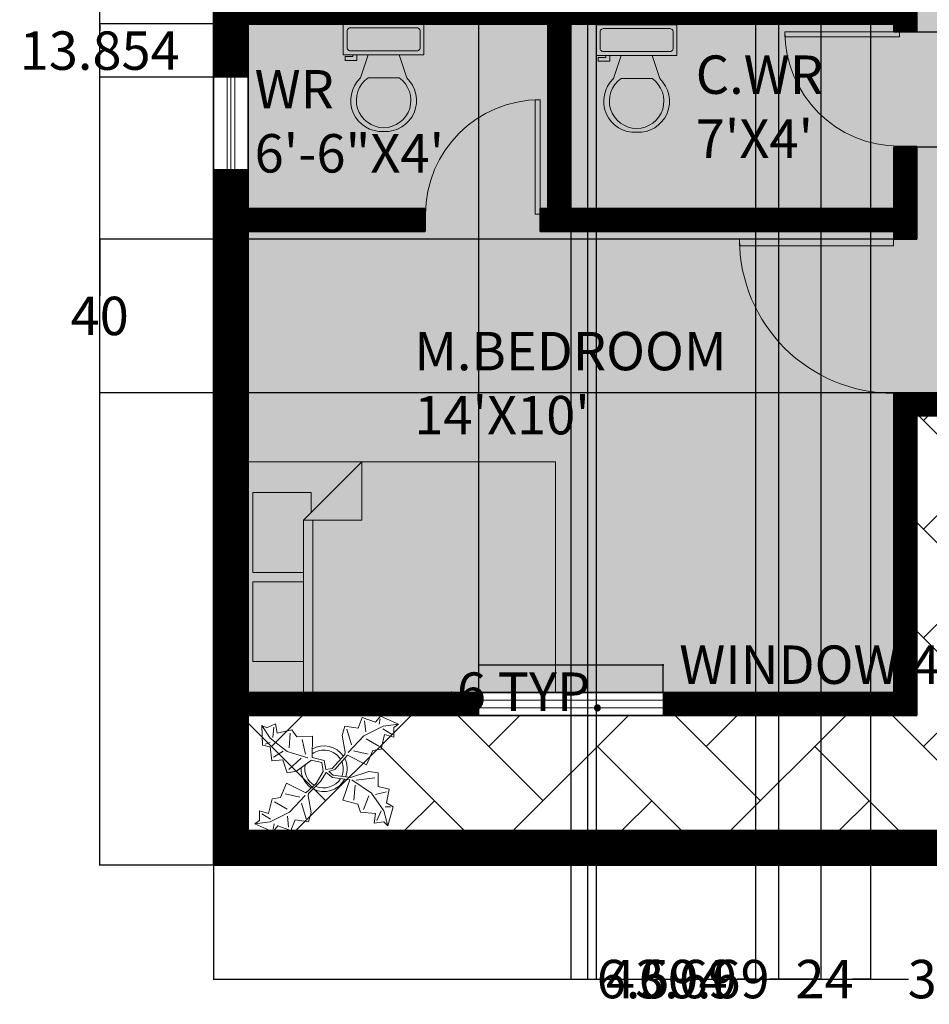
# Model space of a CAD drawing. Units: inches. Extents: x -89252 to 1164, y -183799 to 823.
# Tile 1 of 4: x 670 to 907, y 159 to 416. Entities that reach past the tile are written whole.
import ezdxf

# ---------------------------------------------------------------- set-up
doc = ezdxf.new("R2010")
doc.units = ezdxf.units.IN
doc.header["$MEASUREMENT"] = 0
for name, color, linetype, lineweight in [('A-ANNO-DIMS', 2, 'Continuous', 18), ('A-AREA-IDEN', 7, 'Continuous', 25), ('A-GLAZ', 4, 'Continuous', 18), ('A-WALL', 7, 'Continuous', 35), ('BED', 7, 'Continuous', 18), ('DOOR', 7, 'Continuous', 18), ('PLANT', 3, 'Continuous', 13), ('TOILET', 7, 'Continuous', 18)]:
    doc.layers.add(name, color=color, linetype=linetype, lineweight=lineweight)
for name, color, linetype, lineweight, true_color in [('A-FLOR-PATT', 252, 'Continuous', 13, 0x939598), ('A-WALL-PATT', 18, 'Continuous', 13, 0x000000), ('L-PVMT-PATT', 51, 'Continuous', 13, 0xf8f6b0)]:
    doc.layers.add(name, color=color, linetype=linetype, lineweight=lineweight, true_color=true_color)
doc.styles.get("Standard").update_dxf_attribs({"font": 'arial.ttf'})
doc.dimstyles.get("Standard").update_dxf_attribs({"dimtxt": 10, "dimasz": 0.18, "dimexe": 0.18, "dimexo": 0.0625, "dimgap": 0.09, "dimtad": 0, "dimtih": 1, "dimtoh": 1, "dimdec": 0, "dimzin": 0, "dimdsep": 46, "dimlunit": 3, "dimtxsty": 'Standard', "dimcen": 0.09, "dimadec": 0, "dimazin": 0, "dimtfac": 1, "dimtdec": 0, "dimtofl": 0, "dimtmove": 0, "dimatfit": 3, "dimfxl": 1, "dimtolj": 1, "dimtzin": 0, "dimarcsym": 0})

# ---------------------------------------------------------------- blocks, each defined once
blk = doc.blocks.new('*U5')
for p, q in [((0, 0), (0, -6)), ((40, 0), (40, -6))]:
    blk.add_line(p, q)
blk.add_lwpolyline([(0, 0), (0, 40), (1.75, 40), (1.75, 0)], close=True)
blk.add_arc((0, 0), 40, 0, 90)
blk = doc.blocks.new('*U6')
for p, q in [((-40, 0), (-40, 6)), ((0, 0), (0, 6))]:
    blk.add_line(p, q)
blk.add_lwpolyline([(0, 0), (0, -40), (-1.75, -40), (-1.75, 0)], close=True)
blk.add_arc((0, 0), 40, 180, 270)
blk = doc.blocks.new('Plant - Rubber or Philodendron')
for p, q in [((8.8871, 10.7908), (9.9809, 13.4933)), ((9.9809, 13.4933), (13.3837, 12.301)), ((13.3837, 12.301), (14.68, 13.9039)), ((14.5816, 13.2037), (14.3848, 11.8033)), ((14.68, 13.9039), (19.3848, 11.8146)), ((-16.2005, 11.4774), (-13.9899, 8.1064)), ((-16.2005, 11.4774), (-14.8639, 10.7964)), ((-16.0159, 6.3329), (-16.2005, 11.4774)), ((-14.8639, 10.7964), (-12.6195, 11.8975)), ((-13.3174, 8.325), (-13.0735, 11.0065)), ((-12.6195, 11.8975), (-12.1909, 9.4345)), ((-12.1909, 9.4345), (-8.3829, 10.3)), ((-8.3829, 10.3), (-7.0549, 8.501)), ((4.6914, 8.8812), (5.3859, 11.2828)), ((5.3859, 11.2828), (8.8871, 10.7908)), ((5.9878, 10.4842), (7.1971, 6.3869)), ((15.3859, 11.3055), (10.3916, 8.7942)), ((10.5828, 12.6946), (10.8893, 9.7953)), ((15.2875, 10.6053), (17.5907, 9.2105)), ((19.3848, 11.8146), (15.3859, 11.3055)), ((19.3848, 11.8146), (18.1868, 10.9119)), ((18.1868, 10.9119), (18.1925, 8.4119)), ((-13.9899, 8.1064), (-9.5434, 4.7185)), ((-8.8369, 9.409), (-9.0894, 5.6095)), ((-7.0549, 8.501), (-3.0284, 8.6941)), ((-4.8529, 4.012), (-5.7184, 7.82)), ((-3.0284, 8.6941), (-3.0709, 3.1041)), ((4.6914, 8.8812), (5.5014, 4.4831)), ((10.3916, 8.7942), (6.2847, 4.4028)), ((14.2977, 6.1031), (10.9934, 7.9956)), ((15.7909, 9.1065), (14.8995, 5.3044)), ((18.1925, 8.4119), (15.7909, 9.1065)), ((-14.0069, 5.8704), (-16.0159, 6.3329)), ((-15.3434, 6.5514), (-13.9984, 6.9884)), ((-13.5868, 2.2894), (-14.0069, 5.8704)), ((14.8995, 5.3044), (12.7005, 4.8994)), ((-13.1329, 3.1804), (-10.6614, 4.727)), ((-9.5434, 4.7185), (-4.1917, 2.9888)), ((-9.1318, 0.0195), (-5.9793, 2.9025)), ((-3.0709, 3.1041), (0.0797, 2.3163)), ((2.1141, 0.2298), (5.4346, 3.9146)), ((6.1032, 3.6844), (2.8262, -0.031)), ((5.4346, 3.9146), (5.5014, 4.4831)), ((11.1089, 1.1958), (6.1032, 3.6844)), ((7.7005, 4.8881), (11.5025, 3.9967)), ((12.7005, 4.8994), (11.1089, 1.1958)), ((-10.6784, 2.491), (-13.5868, 2.2894)), ((-9.5858, -0.8715), (-10.6784, 2.491)), ((-7.1228, -0.443), (-3.5248, 2.2131)), ((-3.5248, 2.2131), (-3.3011, 2.4355)), ((-3.3011, 2.4355), (-0.5306, 1.7947)), ((-0.5306, 1.7947), (-0.2255, -0.5527)), ((-0.5306, 1.7947), (-0.5306, 1.7947)), ((0.0797, 2.3163), (0.4866, -0.031)), ((0.4866, -0.031), (2.1141, 0.2298)), ((-7.1228, -0.443), (-9.5858, -0.8715)), ((-2.019, -3.6148), (-0.2255, -0.5527)), ((-0.9375, -3.1608), (0.5883, -0.8135)), ((0.5883, -0.8135), (2.2447, -2.0916)), ((2.8262, -0.031), (1.3003, -0.5527)), ((1.3003, -0.5527), (2.4193, -1.4655)), ((2.2447, -2.0916), (6.7108, -2.6626)), ((2.4193, -1.4655), (6.895, -2.1175)), ((11.6605, -0.5413), (6.895, -2.1175)), ((8.3544, -2.7453), (13.1973, -2.1704)), ((11.6605, -0.5413), (14.1354, -0.8948)), ((14.1354, -0.8948), (14.1354, -4.4304)), ((-11.3237, -7.2629), (-9.7321, -3.5593)), ((-9.7321, -3.5593), (-4.7264, -6.0479)), ((-2.019, -3.6148), (-4.7264, -6.0479)), ((-4.0579, -6.2781), (-0.9375, -3.1608)), ((4.943, -7.9659), (6.7108, -2.6626)), ((12.3677, -6.1981), (7.219, -2.6772)), ((8.125, -4.0768), (7.7715, -7.9659)), ((14.1354, -4.4304), (16.9638, -5.1375)), ((-14.4141, -11.4699), (-13.5228, -7.6679)), ((-13.5228, -7.6679), (-11.3237, -7.2629)), ((-6.3237, -7.2516), (-10.1257, -6.3602)), ((-9.0148, -11.1577), (-4.9047, -6.8122)), ((-4.1246, -6.8466), (-4.0579, -6.2781)), ((-3.3146, -11.2447), (-4.1246, -6.8466)), ((10.2463, -10.4408), (11.6605, -6.9053)), ((15.5496, -10.7943), (12.3677, -6.1981)), ((16.2567, -5.8446), (13.4283, -6.5517)), ((16.9638, -5.1375), (16.2567, -8.673)), ((-12.921, -8.4665), (-9.6166, -10.359)), ((-4.611, -12.8477), (-5.8203, -8.7504)), ((8.8321, -9.0266), (4.943, -7.9659)), ((9.5392, -11.1479), (8.8321, -9.0266)), ((17.3174, -9.7337), (15.9032, -9.7337)), ((16.2567, -8.673), (18.0245, -9.7337)), ((18.0245, -9.7337), (16.6103, -14.6834)), ((-16.8157, -10.7754), (-14.4141, -11.4699)), ((-16.8101, -13.2754), (-16.8157, -10.7754)), ((-13.9107, -12.9688), (-16.2139, -11.574)), ((-14.0091, -13.669), (-9.0148, -11.1577)), ((-9.206, -15.0581), (-9.5126, -12.1588)), ((-3.3146, -11.2447), (-4.0092, -13.6463)), ((13.4283, -11.5015), (9.5392, -11.1479)), ((13.0748, -13.9763), (13.4283, -11.5015)), ((14.8425, -10.7943), (13.7819, -13.2692)), ((16.6103, -14.6834), (15.5496, -10.7943)), ((-18.008, -14.1781), (-16.8101, -13.2754)), ((-18.008, -14.1781), (-14.0091, -13.669)), ((-13.3032, -16.2674), (-18.008, -14.1781)), ((-12.0069, -14.6645), (-13.3032, -16.2674)), ((-13.2048, -15.5672), (-13.008, -14.1668)), ((-8.6042, -15.8568), (-12.0069, -14.6645)), ((-7.5103, -13.1543), (-8.6042, -15.8568)), ((-4.0092, -13.6463), (-7.5103, -13.1543)), ((15.5496, -13.6228), (13.0748, -13.9763)), ((16.6103, -14.6834), (15.5496, -13.6228))]:
    blk.add_line(p, q)
for centre, radius, start, end in [((0, 0), 6.1275, 34.37569, 120.1028), ((-0.0601, -0.2075), 5.2461, 33.82192, 124.9414), ((-0.098, 0.1364), 6.1288, 341.2017, 26.09184), ((0.0308, 0.1664), 6, 178.6147, 235.1169), ((0.0308, 0.1664), 5, 168.1647, 238.6725), ((-0.2664, 0.1682), 5.2775, 338.4094, 20.03007), ((-0.1102, 0.4886), 5.2883, 247.3711, 327.472), ((-0.0234, 0.3825), 6.1492, 242.5812, 331.2714)]:
    blk.add_arc(centre, radius, start, end)
blk = doc.blocks.new('Bed - Queen')
for p, q in [((0, -80.00003), (0, 0)), ((0, 0), (59.99999, 0)), ((59.99999, 0), (59.99999, -80.00003)), ((7.99999, -1.2), (28.79998, -1.2)), ((7.99999, -14.4), (7.99999, -1.2)), ((28.79998, -1.2), (28.79998, -14.4)), ((31.19999, -1.2), (51.99999, -1.2)), ((31.19999, -14.4), (31.19999, -1.2)), ((51.99999, -1.2), (51.99999, -16.4)), ((0, -14.4), (44.8, -14.4)), ((59.99999, -29.6), (44.8, -14.4)), ((44.8, -14.4), (44.8, -29.6)), ((44.8, -16.8), (0, -16.8)), ((51.99999, -16.4), (46.79936, -16.4)), ((44.8, -29.6), (59.99999, -29.6)), ((59.99999, -80.00003), (0, -80.00003))]:
    blk.add_line(p, q)
blk = doc.blocks.new('*U12')
for p, q in [((9.5, -6), (9.5, -2)), ((-10, -8.5), (-8, -8.5)), ((-10, -9.5), (-10, -8.5)), ((-7, -9.5), (-10, -9.5)), ((-8, -8.5), (-8, -8)), ((-7, -8), (-7, -9.5)), ((-4, -8), (-6, -14)), ((4, -8), (6, -14)), ((4, -14), (-4, -14))]:
    blk.add_line(p, q)
blk.add_lwpolyline([(10.5, -8), (10.5, 0), (-10.5, 0), (-10.5, -8)], close=True)
for points in [[(-9.5, -2), (-9.5, -6)], [(8.5, -1), (-8.5, -1)], [(-8.5, -7), (8.5, -7)]]:
    blk.add_lwpolyline(points)
for centre, radius, start, end in [((-8.625, -1.875), 0.8839, 81.8699, 188.1301), ((8.625, -1.875), 0.8839, 351.8699, 98.1301), ((-8.625, -6.125), 0.8839, 171.869898, 278.1301), ((8.625, -6.125), 0.8839, 261.8699, 8.1301), ((-0.4772, -19.9188), 8.0953, 133.01722, 273.38), ((0.0374, -19.8731), 7.127, 124.50543, 269.7), ((-0.0373, -19.8731), 7.127, 270.3, 55.4946), ((0.4773, -19.9188), 8.0953, 266.62, 46.9828)]:
    blk.add_arc(centre, radius, start, end)
blk = doc.blocks.new('WIN-24IN-9IN-WALL')
for p, q in [((9, 24), (0, 24)), ((3.5, 0), (3.5, 24)), ((4.5, 0), (4.5, 24)), ((5.5, 0), (5.5, 24)), ((9, 0), (0, 0))]:
    blk.add_line(p, q)
blk = doc.blocks.new('WIN-48IN-6IN-WALL')
for p, q in [((0, 0), (0, 6)), ((48, 0), (48, 6)), ((0, 4), (48, 4)), ((0, 2), (48, 2))]:
    blk.add_line(p, q)
blk = doc.blocks.new('*D22')
at = {"layer": 'A-ANNO-DIMS', "color": 0, "lineweight": -2, "transparency": 16777216}
for p, q in [((789.36, 240.45), (789.36, 247.77)), ((789.54, 247.59), (837.18, 247.59)), ((837.36, 240.45), (837.36, 247.77)), ((837.36, 247.59), (837.54, 247.59))]:
    blk.add_line(p, q, dxfattribs=at)
at = {"layer": 'A-ANNO-DIMS', "color": 0, "transparency": 16777216}
for points in [[(789.54, 247.62), (789.54, 247.56), (789.36, 247.59)], [(837.18, 247.62), (837.18, 247.56), (837.36, 247.59)]]:
    blk.add_solid(points, dxfattribs=at)
at = {"layer": 'Defpoints', "color": 0, "transparency": 16777216}
for p in [(837.36, 247.59), (789.36, 240.39), (837.36, 240.39)]:
    blk.add_point(p, dxfattribs=at)
at = {"layer": 'A-ANNO-DIMS', "color": 0, "transparency": 16777216, "insert": (894.77, 247.59), "char_height": 10, "attachment_point": 5}
blk.add_mtext('\\A1;WINDOW 48 TYP.', dxfattribs=at)
blk = doc.blocks.new('*D23')
at = {"layer": 'A-ANNO-DIMS', "color": 0, "lineweight": -2, "transparency": 16777216}
for p, q in [((789.3, 240.39), (781.98, 240.39)), ((782.16, 240.39), (782.16, 240.57)), ((782.16, 240.57), (782.34, 240.57)), ((782.16, 234.57), (782.16, 240.21)), ((789.3, 234.39), (781.98, 234.39))]:
    blk.add_line(p, q, dxfattribs=at)
at = {"layer": 'A-ANNO-DIMS', "color": 0, "transparency": 16777216}
for points in [[(782.13, 240.21), (782.19, 240.21), (782.16, 240.39)], [(782.13, 234.57), (782.19, 234.57), (782.16, 234.39)]]:
    blk.add_solid(points, dxfattribs=at)
at = {"layer": 'Defpoints', "color": 0, "transparency": 16777216}
for p in [(782.16, 240.39), (789.36, 240.39), (789.36, 234.39)]:
    blk.add_point(p, dxfattribs=at)
at = {"layer": 'A-ANNO-DIMS', "color": 0, "transparency": 16777216, "insert": (802.91, 240.57), "char_height": 10, "attachment_point": 5}
blk.add_mtext('\\A1;6 TYP.', dxfattribs=at)
blk = doc.blocks.new('*D30')
at = {"layer": 'A-ANNO-DIMS', "color": 0, "lineweight": -2, "transparency": 16777216}
for p, q in [((720.36, 195.33), (720.36, 165.56)), ((1104.36, 195.33), (1104.36, 165.56)), ((720.54, 165.74), (901.25, 165.74)), ((1104.18, 165.74), (923.48, 165.74))]:
    blk.add_line(p, q, dxfattribs=at)
at = {"layer": 'A-ANNO-DIMS', "color": 0, "transparency": 16777216}
for points in [[(720.54, 165.77), (720.54, 165.71), (720.36, 165.74)], [(1104.18, 165.77), (1104.18, 165.71), (1104.36, 165.74)]]:
    blk.add_solid(points, dxfattribs=at)
at = {"layer": 'Defpoints', "color": 0, "transparency": 16777216}
for p in [(720.36, 195.39), (1104.36, 195.39), (1104.36, 165.74)]:
    blk.add_point(p, dxfattribs=at)
at = {"layer": 'A-ANNO-DIMS', "color": 0, "transparency": 16777216, "insert": (912.36, 165.74), "char_height": 10, "attachment_point": 5}
blk.add_mtext('\\A1;384', dxfattribs=at)
blk = doc.blocks.new('*D31')
at = {"layer": 'A-ANNO-DIMS', "color": 0, "lineweight": -2, "transparency": 16777216}
for p, q in [((720.3, 735.39), (690.53, 735.39)), ((690.71, 735.21), (690.71, 470.59)), ((690.71, 195.57), (690.71, 460.19)), ((720.3, 195.39), (690.53, 195.39))]:
    blk.add_line(p, q, dxfattribs=at)
at = {"layer": 'A-ANNO-DIMS', "color": 0, "transparency": 16777216}
for points in [[(690.68, 735.21), (690.74, 735.21), (690.71, 735.39)], [(690.68, 195.57), (690.74, 195.57), (690.71, 195.39)]]:
    blk.add_solid(points, dxfattribs=at)
at = {"layer": 'Defpoints', "color": 0, "transparency": 16777216}
for p in [(690.71, 735.39), (720.36, 735.39), (720.36, 195.39)]:
    blk.add_point(p, dxfattribs=at)
at = {"layer": 'A-ANNO-DIMS', "color": 0, "transparency": 16777216, "insert": (690.71, 465.39), "char_height": 10, "attachment_point": 5}
blk.add_mtext('\\A1;540', dxfattribs=at)
blk = doc.blocks.new('*D38')
at = {"layer": 'A-ANNO-DIMS', "color": 0, "lineweight": -2, "transparency": 16777216}
for p, q in [((897.3, 358.39), (690.53, 358.39)), ((690.71, 358.21), (690.71, 343.59)), ((690.71, 318.57), (690.71, 333.19)), ((897.3, 318.39), (690.53, 318.39))]:
    blk.add_line(p, q, dxfattribs=at)
at = {"layer": 'A-ANNO-DIMS', "color": 0, "transparency": 16777216}
for points in [[(690.68, 358.21), (690.74, 358.21), (690.71, 358.39)], [(690.68, 318.57), (690.74, 318.57), (690.71, 318.39)]]:
    blk.add_solid(points, dxfattribs=at)
at = {"layer": 'Defpoints', "color": 0, "transparency": 16777216}
for p in [(690.71, 358.39), (897.36, 358.39), (897.36, 318.39)]:
    blk.add_point(p, dxfattribs=at)
at = {"layer": 'A-ANNO-DIMS', "color": 0, "transparency": 16777216, "insert": (690.71, 338.39), "char_height": 10, "attachment_point": 5}
blk.add_mtext('\\A1;40', dxfattribs=at)
blk = doc.blocks.new('*D41')
at = {"layer": 'A-ANNO-DIMS', "color": 0, "lineweight": -2, "transparency": 16777216}
for p, q in [((729.36, 240.45), (729.36, 816.22)), ((729.54, 816.04), (752.1, 816.04)), ((789.18, 816.04), (766.63, 816.04)), ((789.36, 240.45), (789.36, 816.22))]:
    blk.add_line(p, q, dxfattribs=at)
at = {"layer": 'A-ANNO-DIMS', "color": 0, "transparency": 16777216}
for points in [[(729.54, 816.07), (729.54, 816.01), (729.36, 816.04)], [(789.18, 816.07), (789.18, 816.01), (789.36, 816.04)]]:
    blk.add_solid(points, dxfattribs=at)
at = {"layer": 'Defpoints', "color": 0, "transparency": 16777216}
for p in [(789.36, 816.04), (729.36, 240.39), (789.36, 240.39)]:
    blk.add_point(p, dxfattribs=at)
at = {"layer": 'A-ANNO-DIMS', "color": 0, "transparency": 16777216, "insert": (759.36, 816.04), "char_height": 10, "attachment_point": 5}
blk.add_mtext('\\A1;60', dxfattribs=at)
blk = doc.blocks.new('*D44')
at = {"layer": 'A-ANNO-DIMS', "color": 0, "lineweight": -2, "transparency": 16777216}
for p, q in [((867.36, 684.33), (867.36, 165.56)), ((891.36, 684.33), (891.36, 165.56)), ((867.54, 165.74), (872.05, 165.74)), ((891.18, 165.74), (886.68, 165.74))]:
    blk.add_line(p, q, dxfattribs=at)
at = {"layer": 'A-ANNO-DIMS', "color": 0, "transparency": 16777216}
for points in [[(867.54, 165.77), (867.54, 165.71), (867.36, 165.74)], [(891.18, 165.77), (891.18, 165.71), (891.36, 165.74)]]:
    blk.add_solid(points, dxfattribs=at)
at = {"layer": 'Defpoints', "color": 0, "transparency": 16777216}
for p in [(867.36, 684.39), (891.36, 684.39), (891.36, 165.74)]:
    blk.add_point(p, dxfattribs=at)
at = {"layer": 'A-ANNO-DIMS', "color": 0, "transparency": 16777216, "insert": (879.36, 165.74), "char_height": 10, "attachment_point": 5}
blk.add_mtext('\\A1;24', dxfattribs=at)
blk = doc.blocks.new('*D47')
at = {"layer": 'A-ANNO-DIMS', "color": 0, "lineweight": -2, "transparency": 16777216}
for p, q in [((817.67, 690.33), (817.67, 165.56)), ((878.36, 690.33), (878.36, 165.56)), ((817.85, 165.74), (831.02, 165.74)), ((878.18, 165.74), (865.02, 165.74))]:
    blk.add_line(p, q, dxfattribs=at)
at = {"layer": 'A-ANNO-DIMS', "color": 0, "transparency": 16777216}
for points in [[(817.85, 165.77), (817.85, 165.71), (817.67, 165.74)], [(878.18, 165.77), (878.18, 165.71), (878.36, 165.74)]]:
    blk.add_solid(points, dxfattribs=at)
at = {"layer": 'Defpoints', "color": 0, "transparency": 16777216}
for p in [(817.67, 690.39), (878.36, 690.39), (878.36, 165.74)]:
    blk.add_point(p, dxfattribs=at)
at = {"layer": 'A-ANNO-DIMS', "color": 0, "transparency": 16777216, "insert": (848.02, 165.74), "char_height": 10, "attachment_point": 5}
blk.add_mtext('\\A1;60.69', dxfattribs=at)
blk = doc.blocks.new('*D48')
at = {"layer": 'A-ANNO-DIMS', "color": 0, "lineweight": -2, "transparency": 16777216}
for p, q in [((817.67, 684.33), (817.67, 165.56)), ((861.36, 684.33), (861.36, 165.56)), ((817.85, 165.74), (822.34, 165.74)), ((861.18, 165.74), (856.69, 165.74))]:
    blk.add_line(p, q, dxfattribs=at)
at = {"layer": 'A-ANNO-DIMS', "color": 0, "transparency": 16777216}
for points in [[(817.85, 165.77), (817.85, 165.71), (817.67, 165.74)], [(861.18, 165.77), (861.18, 165.71), (861.36, 165.74)]]:
    blk.add_solid(points, dxfattribs=at)
at = {"layer": 'Defpoints', "color": 0, "transparency": 16777216}
for p in [(817.67, 684.39), (861.36, 684.39), (861.36, 165.74)]:
    blk.add_point(p, dxfattribs=at)
at = {"layer": 'A-ANNO-DIMS', "color": 0, "transparency": 16777216, "insert": (839.52, 165.74), "char_height": 10, "attachment_point": 5}
blk.add_mtext('\\A1;43.69', dxfattribs=at)
blk = doc.blocks.new('*D49')
at = {"layer": 'A-ANNO-DIMS', "color": 0, "lineweight": -2, "transparency": 16777216}
for p, q in [((729.3, 414.39), (690.53, 414.39)), ((690.71, 414.21), (690.71, 412.66)), ((729.3, 400.53), (690.53, 400.53)), ((690.71, 400.71), (690.71, 402.26))]:
    blk.add_line(p, q, dxfattribs=at)
at = {"layer": 'A-ANNO-DIMS', "color": 0, "transparency": 16777216}
for points in [[(690.68, 414.21), (690.74, 414.21), (690.71, 414.39)], [(690.68, 400.71), (690.74, 400.71), (690.71, 400.53)]]:
    blk.add_solid(points, dxfattribs=at)
at = {"layer": 'Defpoints', "color": 0, "transparency": 16777216}
for p in [(690.71, 414.39), (729.36, 414.39), (729.36, 400.53)]:
    blk.add_point(p, dxfattribs=at)
at = {"layer": 'A-ANNO-DIMS', "color": 0, "transparency": 16777216, "insert": (690.71, 407.46), "char_height": 10, "attachment_point": 5}
blk.add_mtext('\\A1;13.854', dxfattribs=at)
blk = doc.blocks.new('*D53')
at = {"layer": 'A-ANNO-DIMS', "color": 0, "lineweight": -2, "transparency": 16777216}
for p, q in [((819.96, 414.26), (819.96, 816.22)), ((820.14, 816.04), (824.09, 816.04)), ((840.78, 816.04), (836.83, 816.04)), ((840.96, 414.26), (840.96, 816.22))]:
    blk.add_line(p, q, dxfattribs=at)
at = {"layer": 'A-ANNO-DIMS', "color": 0, "transparency": 16777216}
for points in [[(820.14, 816.07), (820.14, 816.01), (819.96, 816.04)], [(840.78, 816.07), (840.78, 816.01), (840.96, 816.04)]]:
    blk.add_solid(points, dxfattribs=at)
at = {"layer": 'Defpoints', "color": 0, "transparency": 16777216}
for p in [(840.96, 816.04), (819.96, 414.2), (840.96, 414.2)]:
    blk.add_point(p, dxfattribs=at)
at = {"layer": 'A-ANNO-DIMS', "color": 0, "transparency": 16777216, "insert": (830.46, 816.04), "char_height": 10, "attachment_point": 5}
blk.add_mtext('\\A1;21', dxfattribs=at)
blk = doc.blocks.new('*D54')
at = {"layer": 'A-ANNO-DIMS', "color": 0, "lineweight": -2, "transparency": 16777216}
for p, q in [((813.36, 414.33), (813.36, 165.56)), ((819.96, 414.14), (819.96, 165.56)), ((813.54, 165.74), (819.78, 165.74)), ((819.96, 165.74), (820.14, 165.74))]:
    blk.add_line(p, q, dxfattribs=at)
at = {"layer": 'A-ANNO-DIMS', "color": 0, "transparency": 16777216}
for points in [[(813.54, 165.77), (813.54, 165.71), (813.36, 165.74)], [(819.78, 165.77), (819.78, 165.71), (819.96, 165.74)]]:
    blk.add_solid(points, dxfattribs=at)
at = {"layer": 'Defpoints', "color": 0, "transparency": 16777216}
for p in [(813.36, 414.39), (819.96, 414.2), (819.96, 165.74)]:
    blk.add_point(p, dxfattribs=at)
at = {"layer": 'A-ANNO-DIMS', "color": 0, "transparency": 16777216, "insert": (837.11, 165.74), "char_height": 10, "attachment_point": 5}
blk.add_mtext('\\A1;6.594', dxfattribs=at)
blk = doc.blocks.new('*D55')
at = {"layer": 'A-ANNO-DIMS', "color": 0, "lineweight": -2, "transparency": 16777216}
for p, q in [((897.43, 412.39), (1134.19, 412.39)), ((1134.01, 412.21), (1134.01, 402.59)), ((1134.01, 382.57), (1134.01, 392.19)), ((897.43, 382.39), (1134.19, 382.39))]:
    blk.add_line(p, q, dxfattribs=at)
at = {"layer": 'A-ANNO-DIMS', "color": 0, "transparency": 16777216}
for points in [[(1133.98, 412.21), (1134.04, 412.21), (1134.01, 412.39)], [(1133.98, 382.57), (1134.04, 382.57), (1134.01, 382.39)]]:
    blk.add_solid(points, dxfattribs=at)
at = {"layer": 'Defpoints', "color": 0, "transparency": 16777216}
for p in [(897.36, 412.39), (1134.01, 412.39), (897.36, 382.39)]:
    blk.add_point(p, dxfattribs=at)
at = {"layer": 'A-ANNO-DIMS', "color": 0, "transparency": 16777216, "insert": (1134.01, 397.39), "char_height": 10, "attachment_point": 5}
blk.add_mtext('\\A1;30', dxfattribs=at)

msp = doc.modelspace()

# ---------------------------------------------------------------- hatches: boundary and pattern name
at = {"layer": 'A-FLOR-PATT'}
h = msp.add_hatch(color=256, dxfattribs=at)
h.dxf.hatch_style = 1
h.paths.add_polyline_path([(1095.364, 558.3893), (1013.364, 558.3893), (1013.364, 564.3893), (1095.364, 564.3893), (1095.364, 672.3893), (1093.364, 672.3893), (1063.364, 672.3893), (1005.364, 672.3893), (1005.364, 726.3893), (975.364, 726.3893), (975.364, 690.3893), (975.364, 564.3893), (977.364, 564.3893), (977.364, 558.3893), (975.364, 558.3893), (969.364, 558.3893), (967.364, 558.3893), (967.364, 564.3893), (969.364, 564.3893), (969.364, 684.3893), (967.364, 684.3893), (937.364, 684.3893), (891.364, 684.3893), (891.364, 588.3893), (929.3053, 588.3893), (929.3053, 564.3893), (937.364, 564.3893), (937.364, 558.3893), (857.364, 558.3893), (857.364, 564.3893), (861.364, 564.3893), (861.364, 684.3893), (729.364, 684.3893), (729.364, 564.3893), (781.364, 564.3893), (781.364, 558.3893), (729.364, 558.3893), (729.364, 510.3893), (813.364, 510.3893), (813.364, 558.3893), (811.364, 558.3893), (811.364, 564.3893), (813.364, 564.3893), (819.364, 564.3893), (821.364, 564.3893), (821.364, 558.3893), (819.364, 558.3893), (819.364, 510.3893), (859.364, 510.3893), (859.364, 420.3893), (903.364, 420.3893), (903.364, 414.3893), (903.364, 412.3893), (897.364, 412.3893), (897.364, 414.3893), (813.364, 414.3893), (813.364, 366.3893), (897.364, 366.3893), (897.364, 382.3893), (903.364, 382.3893), (903.364, 360.3893), (903.364, 358.3893), (897.364, 358.3893), (897.364, 360.3893), (807.364, 360.3893), (805.364, 360.3893), (805.364, 366.3893), (807.364, 366.3893), (807.364, 414.3893), (729.364, 414.3893), (729.364, 366.3893), (775.364, 366.3893), (775.364, 360.3893), (729.364, 360.3893), (729.364, 240.3893), (897.364, 240.3893), (897.364, 318.3893), (1021.364, 318.3893), (1021.364, 312.3893), (1071.364, 312.3893), (1071.364, 318.3893), (1095.364, 318.3893)])
h.paths.add_polyline_path([(1095.364, 726.3893), (1011.364, 726.3893), (1011.364, 678.3893), (1063.364, 678.3893), (1063.364, 672.3893), (1093.364, 672.3893), (1093.364, 678.3893), (1095.364, 678.3893)])
h.paths.add_polyline_path([(969.364, 726.3893), (729.364, 726.3893), (729.364, 690.3893), (937.364, 690.3893), (937.364, 684.3893), (967.364, 684.3893), (967.364, 690.3893), (969.364, 690.3893)])
at = {"layer": 'A-WALL-PATT'}
h = msp.add_hatch(dxfattribs=at)
h.set_pattern_fill('ANSI31', color=256)
h.paths.add_polyline_path([(867.364, 684.3893), (878.364, 684.3893), (878.364, 690.3893), (817.6735, 690.3893), (817.6735, 684.3893), (861.364, 684.3893), (861.364, 564.3893), (857.364, 564.3893), (857.364, 558.3893), (937.364, 558.3893), (937.364, 564.3893), (867.364, 564.3893)], flags=17)
h.paths.add_polyline_path([(1041.364, 735.3893), (720.364, 735.3893), (720.364, 546.3893), (729.364, 546.3893), (729.364, 558.3893), (781.364, 558.3893), (781.364, 564.3893), (729.364, 564.3893), (729.364, 684.3893), (769.6735, 684.3893), (769.6735, 690.3893), (729.364, 690.3893), (729.364, 726.3893), (969.364, 726.3893), (969.364, 690.3893), (967.364, 690.3893), (967.364, 684.3893), (969.364, 684.3893), (969.364, 564.3893), (967.364, 564.3893), (967.364, 558.3893), (969.364, 558.3893), (975.364, 558.3893), (977.364, 558.3893), (977.364, 564.3893), (975.364, 564.3893), (975.364, 690.3893), (975.364, 726.3893), (1005.364, 726.3893), (1005.364, 672.3893), (1063.364, 672.3893), (1063.364, 678.3893), (1011.364, 678.3893), (1011.364, 726.3893), (1041.364, 726.3893)])
h.paths.add_polyline_path([(1104.364, 735.3893), (1065.364, 735.3893), (1065.364, 726.3893), (1095.364, 726.3893), (1095.364, 678.3893), (1093.364, 678.3893), (1093.364, 672.3893), (1095.364, 672.3893), (1095.364, 642.3893), (1104.364, 642.3893)])
h.paths.add_polyline_path([(1104.364, 594.3893), (1095.364, 594.3893), (1095.364, 564.3893), (1013.364, 564.3893), (1013.364, 558.3893), (1095.364, 558.3893), (1095.364, 515.2697), (1104.364, 515.2697)])
h.paths.add_polyline_path([(1104.364, 467.2697), (1095.364, 467.2697), (1095.364, 419.2348), (1104.364, 419.2348)])
h.paths.add_polyline_path([(1104.364, 371.2348), (1095.364, 371.2348), (1095.364, 312.3893), (1104.364, 312.3893)], flags=17)
h.paths.add_polyline_path([(1095.364, 318.3893), (1071.364, 318.3893), (1071.364, 312.3893), (1095.364, 312.3893)], flags=17)
h.paths.add_polyline_path([(1021.364, 318.3893), (897.364, 318.3893), (897.364, 240.3893), (837.364, 240.3893), (837.364, 234.3893), (903.364, 234.3893), (903.364, 312.3893), (1021.364, 312.3893)], flags=17)
h.paths.add_polyline_path([(903.364, 382.3893), (897.364, 382.3893), (897.364, 366.3893), (813.364, 366.3893), (813.364, 414.3893), (897.364, 414.3893), (897.364, 412.3893), (903.364, 412.3893), (903.364, 414.3893), (903.364, 420.3893), (729.364, 420.3893), (729.364, 504.3893), (859.364, 504.3893), (859.364, 510.3893), (819.364, 510.3893), (819.364, 558.3893), (821.364, 558.3893), (821.364, 564.3893), (819.364, 564.3893), (813.364, 564.3893), (811.364, 564.3893), (811.364, 558.3893), (813.364, 558.3893), (813.364, 510.3893), (729.364, 510.3893), (729.364, 522.3893), (720.364, 522.3893), (720.364, 400.5349), (729.364, 400.5349), (729.364, 414.3893), (807.364, 414.3893), (807.364, 366.3893), (805.364, 366.3893), (805.364, 360.3893), (807.364, 360.3893), (897.364, 360.3893), (897.364, 358.3893), (903.364, 358.3893), (903.364, 360.3893)])
h.paths.add_polyline_path([(775.364, 366.3893), (729.364, 366.3893), (729.364, 376.5349), (720.364, 376.5349), (720.364, 195.3893), (1104.364, 195.3893), (1104.364, 204.3893), (729.364, 204.3893), (729.364, 234.3893), (789.364, 234.3893), (789.364, 240.3893), (729.364, 240.3893), (729.364, 360.3893), (775.364, 360.3893)])
h.paths.add_polyline_path([(937.364, 690.3893), (926.364, 690.3893), (926.364, 684.3893), (937.364, 684.3893)], flags=17)
at = {"layer": 'L-PVMT-PATT'}
h = msp.add_hatch(dxfattribs=at)
h.set_pattern_fill('AR-HBONE', color=256, scale=5)
h.paths.add_polyline_path([(1099.864, 258.3893), (1095.364, 312.3893), (1071.364, 312.3893), (1021.364, 312.3893), (903.364, 312.3893), (903.364, 234.3893), (729.364, 234.3893), (729.364, 204.3893), (1095.364, 204.3893)])

# ---------------------------------------------------------------- linework, layer by layer
at = {"layer": 'A-WALL'}
for p, q in [((720.364, 735.3893), (720.364, 195.3893)), ((903.364, 420.3893), (903.364, 414.3893)), ((729.364, 414.3893), (729.364, 366.3893)), ((807.364, 414.3893), (729.364, 414.3893)), ((807.364, 414.3893), (807.364, 366.3893)), ((897.364, 414.3893), (813.364, 414.3893)), ((813.364, 414.3893), (813.364, 366.3893)), ((897.364, 414.3893), (897.364, 412.3893)), ((903.364, 412.3893), (903.364, 414.3893)), ((897.364, 412.3893), (903.364, 412.3893)), ((903.364, 382.3893), (897.364, 382.3893)), ((897.364, 382.3893), (897.364, 366.3893)), ((903.364, 382.3893), (903.364, 360.3893)), ((775.364, 366.3893), (729.364, 366.3893)), ((775.364, 366.3893), (775.364, 360.3893)), ((807.364, 366.3893), (805.364, 366.3893)), ((805.364, 366.3893), (805.364, 360.3893)), ((897.364, 366.3893), (813.364, 366.3893)), ((775.364, 360.3893), (729.364, 360.3893)), ((729.364, 360.3893), (729.364, 240.3893)), ((805.364, 360.3893), (807.364, 360.3893)), ((897.364, 360.3893), (807.364, 360.3893)), ((897.364, 358.3893), (897.364, 360.3893)), ((903.364, 360.3893), (903.364, 358.3893)), ((903.364, 358.3893), (897.364, 358.3893)), ((897.364, 318.3893), (897.364, 240.3893)), ((897.364, 318.3893), (1021.364, 318.3893)), ((903.364, 312.3893), (1021.364, 312.3893)), ((903.364, 312.3893), (903.364, 234.3893)), ((729.364, 240.3893), (897.364, 240.3893)), ((729.364, 234.3893), (897.364, 234.3893)), ((729.364, 234.3893), (903.364, 234.3893)), ((729.364, 234.3893), (729.364, 204.3893)), ((729.364, 204.3893), (1104.364, 204.3893)), ((729.364, 204.3893), (897.364, 204.3893)), ((720.364, 195.3893), (1104.364, 195.3893))]:
    msp.add_line(p, q, dxfattribs=at)

# ---------------------------------------------------------------- block references
at = {"layer": 'A-GLAZ', "rotation": 180}
msp.add_blockref('WIN-24IN-9IN-WALL', (729.3641, 400.5352), dxfattribs=at)
at = {"layer": 'A-GLAZ'}
msp.add_blockref('WIN-48IN-6IN-WALL', (789.364, 234.389), dxfattribs=at)
at = {"layer": 'BED', "rotation": 90}
msp.add_blockref('Bed - Queen', (729.364, 240.3893), dxfattribs=at)
at = {"layer": 'DOOR', "rotation": 270}
for p, xscale, yscale, zscale in [((898.8904, 412.3893), -0.7456098286251903, 0.7456098286251903, 0.7456098286251903), ((897.3462, 358.3893), -1.00297295809016, 1.00297295809016, 1.00297295809016)]:
    msp.add_blockref('*U6', p, dxfattribs=dict(at, xscale=xscale, yscale=yscale, zscale=zscale))
at = {"layer": 'DOOR', "xscale": -0.7456098286251903, "yscale": 0.7456098286251903, "zscale": 0.7456098286251903}
msp.add_blockref('*U5', (805.364, 364.863), dxfattribs=at)
at = {"layer": 'PLANT'}
msp.add_blockref('Plant - Rubber or Philodendron', (749.0843, 220.3166), dxfattribs=at)
at = {"layer": 'TOILET'}
for p in [(764.613, 414.3893), (830.4583, 414.1986)]:
    msp.add_blockref('*U12', p, dxfattribs=at)

# ---------------------------------------------------------------- texts
at = {"layer": 'A-AREA-IDEN', "char_height": 10, "attachment_point": 1}
for s, insert in [("C.WR\\P7'X4'", (845.8363, 406.1986)), ('WR\\P6\'-6"X4\'', (731.0256, 402.3916)), ("M.BEDROOM\\P14'X10'", (772.5949, 334.2304))]:
    msp.add_mtext_dynamic_manual_height_columns(s, width=99.889598, gutter_width=1, heights=[0], dxfattribs=dict(at, insert=insert))

# ---------------------------------------------------------------- dimensions: what is measured, and where the dimension line sits
at = {"layer": 'A-ANNO-DIMS'}
for base, p1, p2, override, picture, middle in [((789.364, 816.0393), (729.364, 240.3893), (789.364, 240.3893), {"dimdec": 0, "dimlfac": 1, "dimrnd": 0, "dimzin": 0, "dimdsep": 46, "dimlunit": 2}, '*D41', (759.364, 816.0393)), ((840.9583, 816.0393), (819.9583, 414.1986), (840.9583, 414.1986), {"dimdec": 0, "dimlfac": 1, "dimrnd": 0, "dimzin": 0, "dimdsep": 46, "dimlunit": 2}, '*D53', (830.4583, 816.0393)), ((878.364, 165.7393), (817.6735, 690.3893), (878.364, 690.3893), {"dimdec": 2, "dimlfac": 1, "dimrnd": 0, "dimzin": 0, "dimdsep": 46, "dimlunit": 2}, '*D47', (848.0188, 165.7393)), ((861.364, 165.7393), (817.6735, 684.3893), (861.364, 684.3893), {"dimdec": 2, "dimlfac": 1, "dimrnd": 0, "dimzin": 0, "dimdsep": 46, "dimlunit": 2}, '*D48', (839.5188, 165.7393)), ((891.364, 165.7393), (867.364, 684.3893), (891.364, 684.3893), {"dimdec": 0, "dimlfac": 1, "dimrnd": 0, "dimzin": 0, "dimdsep": 46, "dimlunit": 2}, '*D44', (879.364, 165.7393)), ((819.9583, 165.7393), (813.364, 414.3893), (819.9583, 414.1986), {"dimdec": 3, "dimlfac": 1, "dimrnd": 0, "dimzin": 0, "dimdsep": 46, "dimlunit": 2}, '*D54', (837.1076, 165.7393)), ((1104.364, 165.7393), (720.364, 195.3893), (1104.364, 195.3893), {"dimdec": 0, "dimlfac": 1, "dimrnd": 0, "dimzin": 0, "dimdsep": 46, "dimlunit": 2}, '*D30', (912.364, 165.7393))]:
    dim = msp.add_linear_dim(base=base, p1=p1, p2=p2, dimstyle='Standard', override=override, dxfattribs=at)
    dim.commit()
    dim.dimension.update_dxf_attribs({"geometry": picture, "text_midpoint": middle})
for base, p1, p2, override, picture, middle in [((690.714, 735.3893), (720.364, 195.3893), (720.364, 735.3893), {"dimdec": 0, "dimlfac": 1, "dimrnd": 0, "dimzin": 0, "dimdsep": 46, "dimlunit": 2}, '*D31', (690.714, 465.3893)), ((690.714, 414.3893), (729.364, 400.5349), (729.364, 414.3893), {"dimdec": 3, "dimlfac": 1, "dimrnd": 0, "dimzin": 0, "dimdsep": 46, "dimlunit": 2}, '*D49', (690.714, 407.4621)), ((1134.014, 412.3893), (897.364, 382.3893), (897.364, 412.3893), {"dimdec": 0, "dimlfac": 1, "dimrnd": 0, "dimzin": 0, "dimdsep": 46, "dimlunit": 2}, '*D55', (1134.014, 397.3893)), ((690.714, 358.3893), (897.364, 318.3893), (897.364, 358.3893), {"dimdec": 0, "dimlfac": 1, "dimrnd": 0, "dimzin": 0, "dimdsep": 46, "dimlunit": 2}, '*D38', (690.714, 338.3893))]:
    dim = msp.add_linear_dim(base=base, p1=p1, p2=p2, angle=90, dimstyle='Standard', override=override, dxfattribs=at)
    dim.commit()
    dim.dimension.update_dxf_attribs({"geometry": picture, "text_midpoint": middle})
dim = msp.add_linear_dim(base=(837.364, 247.5893), p1=(789.364, 240.3893), p2=(837.364, 240.3893), text='WINDOW <> TYP.', dimstyle='Standard', override={"dimdec": 0, "dimlfac": 1, "dimrnd": 0, "dimzin": 0, "dimdsep": 46, "dimlunit": 2}, dxfattribs=at)
dim.commit()
dim.dimension.update_dxf_attribs({"geometry": '*D22', "text_midpoint": (894.7657, 247.5893)})
dim = msp.add_linear_dim(base=(782.164, 240.3893), p1=(789.364, 234.3893), p2=(789.364, 240.3893), angle=90, text='<> TYP.', dimstyle='Standard', override={"dimdec": 0, "dimlfac": 1, "dimrnd": 0, "dimzin": 0, "dimdsep": 46, "dimlunit": 2}, dxfattribs=at)
dim.commit()
dim.dimension.update_dxf_attribs({"geometry": '*D23', "text_midpoint": (802.9149, 240.5693)})

doc.saveas('drawing.dxf')
